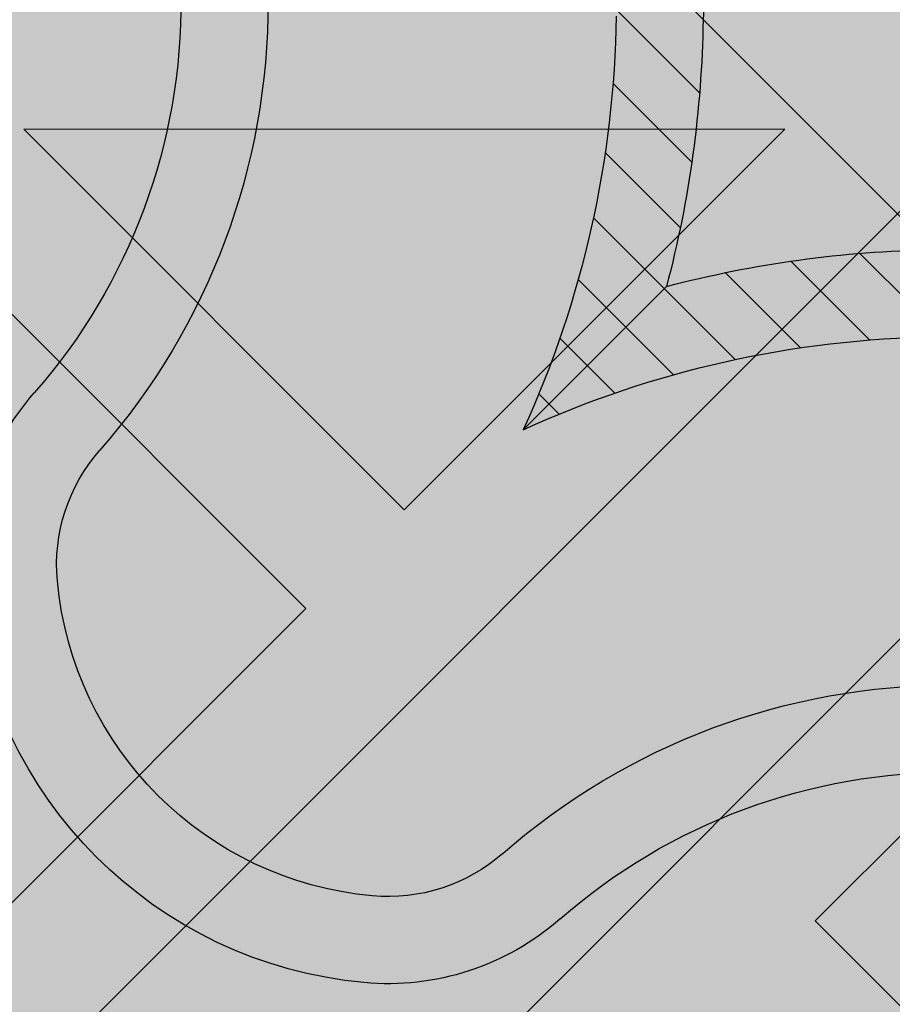
# Model space of a CAD drawing. Units: inches. Extents: x 844 to 2234, y 346 to 1084.
# Tile 70 of 93: x 1999.568 to 2001.166, y 692.525 to 694.327. Entities that reach past the tile are written whole.
import ezdxf

# ---------------------------------------------------------------- set-up
doc = ezdxf.new("R2010")
doc.units = ezdxf.units.IN
doc.header["$MEASUREMENT"] = 0
for name, color, linetype, lineweight in [('A-ANNO-DIMS', 2, 'Continuous', 18), ('furniture', 8, 'Continuous', 18), ('RA-AP-01$0$INT', 35, 'Continuous', 5)]:
    doc.layers.add(name, color=color, linetype=linetype, lineweight=lineweight)
doc.layers.add('RA-AP-01$0$FURN', color=3, linetype='Continuous')
doc.layers.add('RA-AP-01$0$WOOD', color=64, linetype='Continuous')
doc.styles.get("Standard").update_dxf_attribs({"font": 'arial.ttf'})
doc.dimstyles.get("Standard").update_dxf_attribs({"dimtxt": 6, "dimasz": 3, "dimexe": 0.18, "dimexo": 0.0625, "dimgap": 0.09, "dimtad": 0, "dimtih": 1, "dimtoh": 1, "dimdec": 1, "dimzin": 0, "dimdsep": 46, "dimlunit": 3, "dimtxsty": 'Standard', "dimblk": 'ARCHTICK', "dimcen": 0.09, "dimadec": 0, "dimazin": 0, "dimtfac": 1, "dimtdec": 1, "dimtofl": 0, "dimtmove": 0, "dimatfit": 3, "dimfxl": 1, "dimtolj": 1, "dimtzin": 0, "dimarcsym": 0})

# ---------------------------------------------------------------- blocks, each defined once
blk = doc.blocks.new('A$C18D01794')
at = {"layer": 'RA-AP-01$0$INT'}
h = blk.add_hatch(color=256, dxfattribs=at)
h.paths.add_polyline_path([(4.585917135068449, -6.356712009588271), (4.555206456959269, -6.35671200958746), (4.555206456959137, -6.387422687716308), (4.874495778835233, -6.706712009592356), (4.90520645695423, -6.676001331474049)])
h.paths.add_polyline_path([(5.255206456948813, -6.387422687716306), (5.255206456948682, -6.356712009605972), (5.224495778822613, -6.356712009605161), (4.905206456953498, -6.676001331474273), (4.935917135072151, -6.706712009592924)])
h.paths.add_polyline_path([(4.935917135072559, -6.706712009592068), (4.905206456953564, -6.737422687710376), (5.255206456951813, -7.087422687708613), (5.255206456951549, -7.026001331471008)])
h.paths.add_polyline_path([(4.555206456956399, -7.026001331471013), (4.555206456956134, -7.087422687708616), (4.905206456953821, -6.737422687710943), (4.874495778835166, -6.70671200959229)])
h = blk.add_hatch(color=256, dxfattribs=at)
h.paths.add_polyline_path([(4.585917135068448, -6.356712009588273), (4.614201406330596, -6.356712009589021), (4.668846067270487, -6.411356670531338), (4.723490728212344, -6.356712009591912), (4.771774999457151, -6.35671200959319), (4.826419660396886, -6.411356670535356), (4.862780050090322, -6.374996280843536), (4.844495778842715, -6.356712009595112), (4.862780050090411, -6.356712009595595), (4.905206456960182, -6.399138416468211), (4.947632863832445, -6.356712009597838), (4.965917135079675, -6.356712009598322), (4.947632863831759, -6.374996280845421), (4.983993253523576, -6.411356670538857), (5.038637914464627, -6.356712009600247), (5.08692218571208, -6.356712009601523), (5.141566846649976, -6.411356670541852), (5.196211507589851, -6.356712009604411), (5.224495778822615, -6.356712009605161), (4.905206456953975, -6.676001331473793)])
h.paths.add_polyline_path([(4.895206456956031, -6.637717060225675), (4.895206456958921, -6.528427738347902), (4.840561796018589, -6.583072399285802)], flags=16)
h.paths.add_polyline_path([(4.915206456955638, -6.637717060226121), (4.969851117895509, -6.583072399288678), (4.915206456957609, -6.528427738348344)], flags=16)
h.paths.add_polyline_path([(4.826419660395175, -6.568930263661755), (4.881064321335613, -6.514285602723745), (4.771774999456703, -6.514285602720857)], flags=16)
h.paths.add_polyline_path([(4.983993253519558, -6.568930263665262), (5.038637914460456, -6.514285602726792), (4.929348592581548, -6.514285602724816)], flags=16)
h.paths.add_polyline_path([(4.881064321336025, -6.494285602723742), (4.826419660397532, -6.439640941782821), (4.771774999457062, -6.494285602720859)], flags=16)
h.paths.add_polyline_path([(4.929348592582019, -6.494285602724817), (5.038637914460982, -6.494285602726792), (4.983993253522945, -6.439640941786327)], flags=16)
h.paths.add_polyline_path([(4.895206456960191, -6.480143467100443), (4.895206456962115, -6.407422687715913), (4.876922185715016, -6.389138416467584), (4.840561796021581, -6.425498806159401)], flags=16)
h.paths.add_polyline_path([(4.915206456958487, -6.480143467100889), (4.969851117899527, -6.425498806162279), (4.933490728206909, -6.389138416468043), (4.9152064569598, -6.40742268771434)], flags=16)
h.paths.add_polyline_path([(4.757632863832376, -6.480143467096812), (4.812277524772842, -6.425498806158772), (4.757632863834348, -6.370854145217844)], flags=16)
h.paths.add_polyline_path([(4.737632863832376, -6.480143467096286), (4.737632863834348, -6.370854145217375), (4.682988202893906, -6.425498806155385)], flags=16)
h.paths.add_polyline_path([(5.05278005008503, -6.480143467103376), (5.052780050087917, -6.370854145224413), (4.998135389146995, -6.425498806162908)], flags=16)
h.paths.add_polyline_path([(5.072780050085024, -6.480143467103744), (5.127424711025931, -6.42549880616527), (5.072780050087916, -6.370854145224832)], flags=16)
h.paths.add_polyline_path([(4.935917135072783, -6.706712009592292), (5.255206456948811, -6.387422687716309), (5.255206456948932, -6.415706958964177), (5.200561796010279, -6.470351619902839), (5.255206456949403, -6.524996280841948), (5.25520645694961, -6.5732805520894), (5.200561796009787, -6.627925213029239), (5.236922185702417, -6.664285602721864), (5.255206456949919, -6.646001331474357), (5.255206456949998, -6.664285602721898), (5.212780050078687, -6.706712009592262), (5.25520645695036, -6.749138416463932), (5.255206456950438, -6.767422687711313), (5.236922185702424, -6.749138416463297), (5.200561796009796, -6.785498806155928), (5.255206456950753, -6.840143467096874), (5.25520645695096, -6.888427738341682), (5.200561796010322, -6.943072399282328), (5.255206456951428, -6.997717060223427), (5.255206456951547, -7.026001331471006)])
h.paths.add_polyline_path([(5.042988202883395, -6.785498806155427), (5.097632863823085, -6.840143467095101), (5.097632863822622, -6.730854145216193)], flags=16)
h.paths.add_polyline_path([(5.028846067259663, -6.771356670531693), (5.083490728198774, -6.716712009592573), (4.974201406321001, -6.716712009593042)], flags=16)
h.paths.add_polyline_path([(5.117632863823087, -6.840143467095186), (5.172277524762331, -6.785498806155926), (5.11763286382262, -6.730854145216225)], flags=16)
h.paths.add_polyline_path([(5.08349072819877, -6.696712009593886), (5.028846067259652, -6.642067348654775), (4.974201406320998, -6.696712009593438)], flags=16)
h.paths.add_polyline_path([(5.131774999446817, -6.854285602718917), (5.186419660386065, -6.799640941779662), (5.241064321325782, -6.854285602719365)], flags=17)
h.paths.add_polyline_path([(5.131774999446228, -6.716712009592374), (5.186419660386065, -6.771356670532194), (5.222780050079488, -6.734996280838764), (5.204495778832781, -6.716712009592063)], flags=16)
h.paths.add_polyline_path([(5.097632863822613, -6.682569873970264), (5.097632863823061, -6.573280552091354), (5.042988202883383, -6.627925213031044)], flags=16)
h.paths.add_polyline_path([(5.131774999446899, -6.874285602718915), (5.241064321325809, -6.874285602719364), (5.186419660386591, -6.928930263658598)], flags=17)
h.paths.add_polyline_path([(5.131774999446226, -6.696712009594078), (5.204495778830767, -6.696712009594374), (5.22278005007868, -6.67842773834687), (5.186419660386049, -6.642067348654249)], flags=16)
h.paths.add_polyline_path([(5.11763286382262, -6.682569873970225), (5.17227752476232, -6.627925213030515), (5.117632863823064, -6.573280552091267)], flags=16)
h.paths.add_polyline_path([(5.186419660386069, -6.613783077405491), (5.241064321325754, -6.559138416465795), (5.131774999446791, -6.559138416466263)], flags=16)
h.paths.add_polyline_path([(5.131774999446872, -6.539138416466263), (5.24106432132578, -6.539138416465794), (5.186419660386554, -6.484493755526573)], flags=16)
h.paths.add_polyline_path([(5.255206456951811, -7.08742268770861), (5.255206456951895, -7.106712009588038), (4.555206456956052, -7.106712009588038), (4.555206456956136, -7.087422687708617), (4.905206456953973, -6.737422687710788)])
h.paths.add_polyline_path([(4.983993253513404, -6.8444937555241), (4.92934859257295, -6.899138416462108), (5.03863791445186, -6.899138416465014)], flags=16)
h.paths.add_polyline_path([(4.969851117889988, -6.83035161990006), (4.915206456952556, -6.775706958960171), (4.915206456949648, -6.884996280837944)], flags=16)
h.paths.add_polyline_path([(4.929348592572535, -6.919138416462105), (4.983993253511019, -6.973783077403037), (5.038637914451496, -6.919138416465012)], flags=16)
h.paths.add_polyline_path([(5.052780050074912, -6.93328055208906), (4.998135389134438, -6.987925213027088), (5.052780050072919, -7.042569873968025)], flags=16)
h.paths.add_polyline_path([(5.07278005007491, -6.933280552089588), (5.072780050072918, -7.042569873968497), (5.127424711013374, -6.987925213030498)], flags=16)
h.paths.add_polyline_path([(4.89520645695295, -6.775706958959721), (4.840561796013067, -6.830351619897157), (4.895206456950961, -6.884996280837494)], flags=16)
h.paths.add_polyline_path([(4.915206456948365, -6.933280552085403), (4.915206456946434, -7.006001331471951), (4.933490728192729, -7.024285602719066), (4.969851117886972, -6.987925213026453)], flags=16)
h.paths.add_polyline_path([(4.881064321327021, -6.899138416461022), (4.82641966038902, -6.84449375552057), (4.771774999448108, -6.899138416459029)], flags=16)
h.paths.add_polyline_path([(4.895206456950073, -6.933280552084951), (4.840561796009022, -6.987925213023558), (4.876922185700835, -7.024285602716997), (4.895206456948749, -7.006001331469487)], flags=16)
h.paths.add_polyline_path([(4.983993253510392, -7.0020673486505), (4.947632863816944, -7.038427738342319), (4.965917135064043, -7.05671200959023), (5.038637914448995, -7.056712009591555)], flags=16)
h.paths.add_polyline_path([(4.881064321326543, -6.91913841646102), (4.771774999447578, -6.919138416459031), (4.826419660385607, -6.973783077399508)], flags=16)
h.paths.add_polyline_path([(4.905206456946447, -7.014285602717636), (4.862780050074785, -7.056712009588352), (4.947632863816685, -7.056712009589775)], flags=16)
h.paths.add_polyline_path([(5.14156684663679, -7.002067348654549), (5.086922185696452, -7.056712009592438), (5.196211507574223, -7.056712009594425)], flags=16)
h.paths.add_polyline_path([(4.8264196603837, -7.002067348646972), (4.771774999442643, -7.056712009585575), (4.8444957788276, -7.056712009587508), (4.862780050075511, -7.038427738340416)], flags=16)
h.paths.add_polyline_path([(4.812277524760289, -6.98792521302292), (4.757632863822258, -6.933280552082447), (4.757632863819352, -7.042569873961408)], flags=16)
h.paths.add_polyline_path([(4.73763286382226, -6.933280552082079), (4.682988202881349, -6.987925213020536), (4.737632863819352, -7.04256987396099)], flags=16)
h.paths.add_polyline_path([(4.723490728195188, -7.056712009584289), (4.668846067257299, -7.002067348643949), (4.614201406317417, -7.056712009581383)], flags=16)
h.paths.add_polyline_path([(4.597632863829262, -6.706712009592262), (4.555206456957951, -6.664285602721896), (4.555206456958029, -6.646001331474357), (4.573490728205535, -6.664285602721864), (4.609851117898167, -6.627925213029238), (4.555206456958338, -6.573280552089402), (4.555206456958546, -6.524996280841952), (4.60985111789767, -6.470351619902839), (4.555206456959015, -6.415706958964177), (4.555206456959138, -6.387422687716309), (4.874495778835167, -6.70671200959229), (4.5552064569564, -7.026001331471015), (4.555206456956523, -6.997717060223433), (4.609851117897629, -6.94307239928233), (4.555206456956988, -6.888427738341681), (4.555206456957198, -6.840143467096881), (4.609851117898153, -6.78549880615593), (4.573490728205528, -6.749138416463297), (4.555206456957507, -6.76742268771132), (4.555206456957585, -6.749138416463933)])
h.paths.add_polyline_path([(4.712780050085332, -6.730854145216195), (4.712780050084863, -6.840143467095105), (4.767424711024555, -6.785498806155427)], flags=16)
h.paths.add_polyline_path([(4.726922185709173, -6.716712009592573), (4.781566846648288, -6.771356670531693), (4.836211507586949, -6.716712009593043)], flags=16)
h.paths.add_polyline_path([(4.692780050085327, -6.730854145216225), (4.638135389145619, -6.785498806155928), (4.692780050084865, -6.840143467095185)], flags=16)
h.paths.add_polyline_path([(4.726922185709182, -6.696712009593886), (4.836211507586949, -6.696712009593436), (4.7815668466483, -6.642067348654773)], flags=16)
h.paths.add_polyline_path([(4.678637914461726, -6.71671200959237), (4.605917135075169, -6.716712009592063), (4.587632863828464, -6.734996280838766), (4.623993253521887, -6.771356670532195)], flags=16)
h.paths.add_polyline_path([(4.712780050085336, -6.68256987397026), (4.767424711024568, -6.627925213031042), (4.71278005008489, -6.573280552091352)], flags=16)
h.paths.add_polyline_path([(4.678637914461726, -6.696712009594076), (4.623993253521899, -6.642067348654247), (4.587632863829271, -6.67842773834687), (4.605917135077185, -6.696712009594376)], flags=16)
h.paths.add_polyline_path([(4.692780050085336, -6.682569873970228), (4.692780050084889, -6.573280552091267), (4.638135389145632, -6.627925213030515)], flags=16)
h.paths.add_polyline_path([(4.623993253521885, -6.799640941779662), (4.678637914461131, -6.854285602718915), (4.56934859258217, -6.854285602719365)], flags=17)
h.paths.add_polyline_path([(4.623993253521901, -6.613783077405509), (4.678637914461158, -6.559138416466263), (4.569348592582195, -6.559138416465795)], flags=16)
h.paths.add_polyline_path([(4.678637914461051, -6.874285602718915), (4.623993253521361, -6.928930263658598), (4.569348592582143, -6.874285602719364)], flags=17)
h.paths.add_polyline_path([(4.678637914461076, -6.539138416466263), (4.623993253521399, -6.484493755526573), (4.569348592582167, -6.539138416465796)], flags=16)
h = blk.add_hatch(color=256, dxfattribs=at)
h.paths.add_polyline_path([(4.969851117891331, -6.583072399286455), (4.915206456952669, -6.63771706022511), (4.915206456952222, -6.528427738347337)])
h.paths.add_polyline_path([(4.895206456953064, -6.637717060225108), (4.840561796014413, -6.583072399286448), (4.895206456953533, -6.528427738347335)])
h.paths.add_polyline_path([(4.826419660390684, -6.568930263662714), (4.771774999451003, -6.514285602723024), (4.881064321329913, -6.514285602723489)])
h.paths.add_polyline_path([(4.881064321329884, -6.494285602723492), (4.771774999450921, -6.494285602723024), (4.82641966039018, -6.439640941783778)])
h.paths.add_polyline_path([(4.895206456953734, -6.48014346709988), (4.840561796013912, -6.425498806160046), (4.876922185707337, -6.389138416466622), (4.895206456954043, -6.40742268771333)])
h.paths.add_polyline_path([(4.862780050082808, -6.374996280843689), (4.826419660390178, -6.411356670536314), (4.771774999450351, -6.356712009596481), (4.844495778835303, -6.356712009596181)])
h.paths.add_polyline_path([(4.812277524766446, -6.425498806160041), (4.757632863827191, -6.480143467099289), (4.757632863826741, -6.370854145220329)])
h.paths.add_polyline_path([(4.737632863827191, -6.480143467099214), (4.682988202887508, -6.425498806159518), (4.737632863826743, -6.370854145220299)])
h.paths.add_polyline_path([(4.668846067263777, -6.41135667053579), (4.614201406325123, -6.356712009597128), (4.723490728202894, -6.356712009596675)])
h.paths.add_polyline_path([(4.905206456953846, -6.399138416467422), (4.862780050082654, -6.356712009596229), (4.947632863824561, -6.356712009595756)])
h.paths.add_polyline_path([(4.915206456952028, -6.480143467099882), (4.91520645695173, -6.407422687715346), (4.933490728199234, -6.389138416467428), (4.96985111789186, -6.425498806160055)])
h.paths.add_polyline_path([(5.038637914454841, -6.494285602723048), (4.929348592575874, -6.494285602723497), (4.983993253515593, -6.439640941783787)])
h.paths.add_polyline_path([(4.983993253515065, -6.568930263662725), (4.929348592575849, -6.514285602723495), (5.038637914454755, -6.514285602723045)])
h.paths.add_polyline_path([(5.052780050079843, -6.480143467099317), (4.998135389140595, -6.425498806160058), (5.052780050080309, -6.370854145220356)])
h.paths.add_polyline_path([(4.983993253516868, -6.411356670536324), (4.947632863824241, -6.374996280843694), (4.965917135071747, -6.356712009596188), (5.038637914456701, -6.356712009596504)])
h.paths.add_polyline_path([(5.127424711019533, -6.425498806159557), (5.072780050079843, -6.480143467099239), (5.07278005008031, -6.370854145220326)])
h.paths.add_polyline_path([(5.141566846643269, -6.411356670535829), (5.086922185704154, -6.356712009596707), (5.196211507581929, -6.356712009597176)])
h = blk.add_hatch(color=256, dxfattribs=at)
h.paths.add_polyline_path([(5.028846067259997, -6.642067348655121), (4.974201406321342, -6.696712009593783), (5.083490728199115, -6.69671200959423)])
h.paths.add_polyline_path([(4.974201406321344, -6.716712009593388), (5.028846067260004, -6.771356670532039), (5.083490728199117, -6.716712009592919)])
h.paths.add_polyline_path([(5.042988202883738, -6.785498806155768), (5.097632863823428, -6.840143467095449), (5.097632863822963, -6.73085414521654)])
h.paths.add_polyline_path([(5.117632863822961, -6.730854145216568), (5.117632863823428, -6.840143467095531), (5.172277524762674, -6.785498806156272)])
h.paths.add_polyline_path([(5.131774999446572, -6.716712009592718), (5.186419660386406, -6.77135667053254), (5.222780050079831, -6.734996280839116), (5.204495778833122, -6.716712009592409)])
h.paths.add_polyline_path([(5.236922185702764, -6.749138416463644), (5.200561796010139, -6.785498806156274), (5.255206456949971, -6.840143467096101), (5.255206456950271, -6.76742268771115)])
h.paths.add_polyline_path([(5.186419660386412, -6.799640941780006), (5.131774999447164, -6.854285602719262), (5.241064321326123, -6.854285602719711)])
h.paths.add_polyline_path([(5.131774999447238, -6.874285602719261), (5.186419660386934, -6.928930263658944), (5.241064321326153, -6.874285602719709)])
h.paths.add_polyline_path([(5.200561796010663, -6.943072399282675), (5.255206456949324, -6.997717060221329), (5.255206456949777, -6.888427738343558)])
h.paths.add_polyline_path([(5.21278005007903, -6.706712009592607), (5.255206456950223, -6.749138416463798), (5.255206456950696, -6.664285602721891)])
h.paths.add_polyline_path([(5.13177499944657, -6.696712009594424), (5.204495778831106, -6.696712009594723), (5.222780050079024, -6.678427738347219), (5.186419660386397, -6.642067348654592)])
h.paths.add_polyline_path([(5.117632863823405, -6.573280552091611), (5.117632863822955, -6.682569873970578), (5.172277524762665, -6.627925213030859)])
h.paths.add_polyline_path([(5.042988202883727, -6.627925213031387), (5.097632863822957, -6.682569873970603), (5.097632863823407, -6.573280552091697)])
h.paths.add_polyline_path([(5.131774999447135, -6.559138416466609), (5.186419660386394, -6.613783077405857), (5.241064321326097, -6.559138416466144)])
h.paths.add_polyline_path([(5.200561796010128, -6.627925213029584), (5.236922185702758, -6.664285602722211), (5.255206456950264, -6.646001331474705), (5.255206456949948, -6.573280552089752)])
h.paths.add_polyline_path([(5.186419660386895, -6.484493755526919), (5.131774999447213, -6.539138416466609), (5.241064321326127, -6.539138416466142)])
h.paths.add_polyline_path([(5.200561796010624, -6.470351619903183), (5.255206456949745, -6.524996280842298), (5.255206456949276, -6.415706958964523)])
for p, q in [((4.905206456953975, -6.676001331473793), (5.224495778822613, -6.356712009605161)), ((5.072780050087916, -6.37085414522483), (5.127424711025931, -6.42549880616527)), ((4.935917135072783, -6.706712009592292), (5.255206456948813, -6.387422687716307)), ((5.255206456948934, -6.415706958964177), (5.200561796010281, -6.470351619902839)), ((5.12742471102593, -6.425498806165272), (5.072780050085028, -6.48014346710374)), ((5.255206456949399, -6.524996280841946), (5.200561796010281, -6.470351619902839)), ((5.18641966038655, -6.484493755526575), (5.131774999446872, -6.539138416466263)), ((5.241064321325782, -6.539138416465796), (5.186419660386552, -6.484493755526573)), ((5.131774999446872, -6.539138416466263), (5.241064321325782, -6.539138416465796))]:
    blk.add_line(p, q, dxfattribs=at)
blk = doc.blocks.new('A$C32926AE1')
at = {"layer": 'RA-AP-01$0$WOOD'}
h = blk.add_hatch(color=256, dxfattribs=at)
h.dxf.hatch_style = 1
h.paths.add_polyline_path([(5.157430609644524, 4.573483066760929, -0.1009492694046607), (5.155401577623758, 4.593365984175333, -0.1842662638101597), (5.172249623284174, 4.638795604568598, 0.2056608120311276), (5.179560981299304, 4.661316324430096, 0.3614336704623542), (5.134352340494423, 4.706524965234944, 0.2056608120311297), (5.111831620632933, 4.699213607219793, -0.1842662638101113), (5.066402000239693, 4.682365561559342, -0.1055311479399994), (5.045656153913092, 4.68467289944697, 0.1567636581983829), (4.763886414745334, 4.684672899446966, -0.1055311479399895), (4.743140568418733, 4.68236556155934, -0.1842662638100833), (4.6977109480255, 4.69921360721979, 0.2056608120302612), (4.675190228164109, 4.706524965234949, 0.3614336704708441), (4.629981587358889, 4.66131632442871, 0.2056608120245944), (4.637292945374126, 4.638795604567974, -0.1842662638101024), (4.654140991034615, 4.59336598417475, -0.1009492694055169), (4.652111959013835, 4.573483066760181, 0.021410119221476), (4.629748025606143, 4.156712009541676, 0.0214101192214795), (4.652111959013809, 3.739940952323101, -0.1009492694059586), (4.654140991034615, 3.720058034908448, -0.1842662638100975), (4.637292945374126, 3.674628414515226, 0.2056608120245705), (4.629981587358889, 3.652107694654492, 0.3614336704708879), (4.675190228164113, 3.606899053848249, 0.2056608120302384), (4.697710948025501, 3.614210411863408, -0.1842662638100995), (4.743140568418738, 3.63105845752386, -0.1055311479402541), (4.763886414745388, 3.628751119636215, 0.1567636581983776), (5.045656153913137, 3.628751119636244, -0.1055311479397538), (5.066402000239692, 3.631058457523857, -0.1842662638101067), (5.111831620632931, 3.614210411863407, 0.2056608120310924), (5.134352340494417, 3.606899053848256, 0.3614336704624001), (5.179560981299307, 3.652107694653103, 0.2056608120311314), (5.172249623284175, 3.6746284145146, -0.1842662638101402), (5.155401577623758, 3.72005803490786, -0.1009492694051366), (5.15743060964455, 3.739940952322354, 0.0214101192215073), (5.179794543052287, 4.156712009541468, 0.0214101192215252)])
h.paths.add_polyline_path([(4.639748609479751, 4.156712009541513, 0.0213537860821624), (4.661970494867118, 3.741887061152232, -0.094075836301374), (4.664143710413708, 3.7196126951003, -0.1824818158568985), (4.644813765429836, 3.668037719127816, 0.2056608120245319), (4.639939526753007, 3.653023905887301, 0.3614336704710246), (4.676106439397173, 3.616856993242342, 0.2056608120302234), (4.691120252638095, 3.621731231919122, -0.1824818158602558), (4.742695228611606, 3.641061176902986, -0.1029891339458722), (4.766991894714349, 3.638256818950944, 0.156709409989566), (5.042550673941472, 3.638256818950105, -0.102989133958497), (5.066847340047078, 3.641061176902949, -0.1824818158594995), (5.118422316020358, 3.621731231919103, 0.2056608120311416), (5.133436129261316, 3.616856993242346, 0.3614336704621468), (5.169603041905217, 3.653023905886178, 0.2056608120310986), (5.164728803228477, 3.668037719127177, -0.1824818158565612), (5.145398858244737, 3.719612695099578, -0.0940758363009313), (5.147572073791232, 3.741887061151398, 0.0213537860822023), (5.169793959178681, 4.156712009541451, 0.0213537860822226), (5.147572073791203, 4.571536957931898, -0.0940758363005034), (5.145398858244737, 4.59381132398362, -0.1824818158565587), (5.164728803228476, 4.645386299956021, 0.2056608120311045), (5.169603041905216, 4.66040011319702, 0.3614336704621845), (5.133436129261313, 4.696567025840856, 0.2056608120310773), (5.118422316020359, 4.691692787164098, -0.182481815859508), (5.066847340047078, 4.67236284218025, -0.1029891339584606), (5.04255067394148, 4.675167200133092, 0.156709409989566), (4.766991894714357, 4.675167200132257, -0.1029891339458842), (4.742695228611611, 4.672362842180213, -0.1824818158602725), (4.691120252638095, 4.691692787164077, 0.2056608120302152), (4.676106439397174, 4.696567025840858, 0.3614336704710363), (4.639939526753005, 4.660400113195899, 0.2056608120245495), (4.644813765429837, 4.645386299955384, -0.1824818158568934), (4.664143710413708, 4.593811323982902, -0.0940758363009187), (4.661970494867149, 4.571536957931074, 0.021353786082177)], flags=16)
h.paths.add_polyline_path([(5.129794543052235, 4.432167055276933, -0.0141661062790638), (5.130152669293814, 4.156927903047693, -0.0141661062790647), (5.129794543052234, 3.881688750818433, -0.0785247771143638), (5.10979738006795, 3.755143611847103, 0.0945969212073497), (5.105408519571111, 3.717898134952927, 0.1043170707844957), (5.116074640131521, 3.670385395016088, 0.1043170707864965), (5.068561900193738, 3.681051515576561, 0.09459692119553), (5.031316423304057, 3.676662655080835, -0.1580239521427272), (4.778226145355827, 3.676662655080367, 0.0945969211986668), (4.740980668464973, 3.681051515576592, 0.1043170707882822), (4.693467928526415, 3.670385395015844, 0.1043170707867916), (4.704134049087309, 3.717898134953662, 0.0945969211972894), (4.69974518859162, 3.755143611844042, -0.0785247771163196), (4.679748025606343, 3.881688750818406, -0.0141661062790663), (4.679389899364763, 4.156927903047693, -0.0141661062790672), (4.679748025606343, 4.432167055276998, -0.0785247771163064), (4.699745188591625, 4.55871219425134, 0.094596921197333), (4.704134049087308, 4.595957671141738, 0.1043170707867205), (4.693467928526416, 4.643470411079523, 0.1043170707882628), (4.740980668464965, 4.632804290518776, 0.0945969211988114), (4.778226145355874, 4.637193151015016, -0.158023952142669), (5.031316423304015, 4.637193151014546, 0.0945969211956361), (5.068561900193736, 4.632804290518806, 0.1043170707864979), (5.11607464013152, 4.643470411079278, 0.1043170707844617), (5.105408519571112, 4.595957671142455, 0.0945969212074597), (5.109797380067959, 4.558712194248236, -0.0785247771143467)], flags=0)
h.paths.add_polyline_path([(5.119794532311105, 4.432259799204851, -0.0142000800617244), (5.120156169157484, 4.156927903047701, -0.0142000800617277), (5.119794532311105, 3.881596006890482, -0.0784894509520253), (5.100273383573699, 3.758192358677797, 0.0940138827242913), (5.095413455884425, 3.717477693979438, 0.0606271852308753), (5.099615656341024, 3.686844378806616, 0.0606271852322524), (5.068982341167493, 3.691046579263239, 0.0940138827010453), (5.028267676478798, 3.686186651576848, -0.1580706864508061), (4.781274892180912, 3.686186651576435, 0.0940138827026903), (4.740560227491556, 3.691046579263279, 0.0606271852339895), (4.709926912317155, 3.686844378806508, 0.0606271852329405), (4.714129112773991, 3.717477693980356, 0.094013882701304), (4.709269185087677, 3.758192358669163, -0.0784894509577193), (4.689748036347473, 3.881596006890469, -0.014200080061729), (4.689386399501094, 4.156927903047709, -0.0142000800617217), (4.689748036347473, 4.432259799204808, -0.078489450957724), (4.709269185087651, 4.555663447426125, 0.0940138827014585), (4.714129112773992, 4.596378112114996, 0.0606271852329731), (4.709926912317154, 4.62701142728886, 0.0606271852340196), (4.74056022749157, 4.622809226832087, 0.0940138827024997), (4.781274892180847, 4.627669154518912, -0.1580706864508359), (5.028267676478777, 4.627669154518526, 0.0940138827010946), (5.068982341167492, 4.622809226832129, 0.060627185232254), (5.099615656341024, 4.627011427288751, 0.0606271852308727), (5.095413455884425, 4.59637811211593, 0.0940138827241088), (5.100273383573675, 4.555663447417647, -0.0784894509520978)], flags=0)
h.paths.add_polyline_path([(5.06978912287499, 4.430218106756144, -0.014241683694547), (5.070173729147532, 4.156927903047672, -0.0142416836945458), (5.06978912287499, 3.883637699339223, -0.0800609523125196), (5.052662118612511, 3.773463122773442, 0.0526421978001116), (5.04590916754064, 3.740550867606997, 0.0526421977992423), (5.012996912374707, 3.73379791653534, -0.1583028414718258), (4.796545656286308, 3.73379791653451, 0.0526421978034211), (4.763633401117837, 3.740550867607021, 0.0526421978018622), (4.756880450045755, 3.773463122774558, -0.0800609523117106), (4.739753445783639, 3.883637699339268, -0.0142416836945435), (4.739368839511098, 4.156927903047671, -0.0142416836945477), (4.739753445783639, 4.430218106756155, -0.0800609523116345), (4.75688045004574, 4.540392683320762, 0.052642197801941), (4.763633401117837, 4.573304938488346, 0.0526421978035071), (4.796545656286361, 4.580057889560873, -0.1583028414717561), (5.012996912374669, 4.580057889560039, 0.0526421977993048), (5.04590916754064, 4.57330493848837, 0.0526421978002057), (5.052662118612529, 4.540392683321868, -0.080060952312477)], flags=0)
h.paths.add_polyline_path([(5.049789715110557, 4.43038092723357, -0.0143097550741839), (5.05018085590259, 4.156927903047715, -0.0143097550741854), (5.049789715110558, 3.883474878861827, -0.0800685599149176), (5.03362098255317, 3.779581877367999, 0.0306258898956367), (5.028241146483733, 3.758218888663947, 0.0306258898977031), (5.006878157778253, 3.75283905259408, -0.1583983521624096), (4.802664410878162, 3.752839052594731, 0.0306258898946014), (4.781301422174808, 3.758218888663924, 0.0306258898967912), (4.775921586105202, 3.779581877368794, -0.080068559914251), (4.759752853548071, 3.883474878861786, -0.0143097550741854), (4.759361712756037, 4.156927903047671, -0.0143097550741854), (4.759752853548071, 4.430380927233557, -0.0800685599142479), (4.775921586105193, 4.534273928726546, 0.0306258898968306), (4.781301422174808, 4.555636917431444, 0.0306258898945754), (4.802664410878143, 4.561016753500631, -0.1583983521624168), (5.006878157778244, 4.561016753501291, 0.0306258898977177), (5.028241146483733, 4.555636917431421, 0.0306258898958182), (5.03362098255321, 4.534273928727244, -0.080068559914796)], flags=0)
h.paths.add_polyline_path([(4.999766070382627, 4.428171244713864, -0.0143443147609634), (5.000198441819402, 4.156927903047689, -0.0143443147609612), (4.999766070382627, 3.885684561381556, -0.0784641635803329), (4.987356730658798, 3.799103304488872, -0.1506053783831347), (4.822185837999821, 3.79910330448882, -0.0784641635803318), (4.809776498276007, 3.885684561381509, -0.014344314760963), (4.809344126839227, 4.156927903047677, -0.0143443147609645), (4.809776498276007, 4.428171244713873, -0.0784641635803192), (4.822185837999822, 4.514752501606549, -0.1506053783831338), (4.987356730658798, 4.514752501606494, -0.078464163580285)], flags=0)
h.paths.add_polyline_path([(4.979755254238824, 4.42764379880488, -0.0143772539198268), (4.980205517789977, 4.156927903047693, -0.0143772539198275), (4.979755254238824, 3.886212007290489, -0.0689242507424422), (4.971183264704897, 3.815276770442801, -0.1296645318904179), (4.838359303953726, 3.815276770442746, -0.0689242507424186), (4.829787314419809, 3.886212007290419, -0.0143772539198292), (4.829337050868653, 4.156927903047653, -0.0143772539198325), (4.829787314419809, 4.427643798804946, -0.0689242507424211), (4.838359303953725, 4.498579035652621, -0.1296645318904187), (4.971183264704897, 4.498579035652565, -0.0689242507424401)], flags=0)
h = blk.add_hatch(color=256, dxfattribs=at)
h.dxf.hatch_style = 1
h.paths.add_polyline_path([(5.145398858244737, 4.59381132398362, -0.1824818158565616), (5.164728803228476, 4.645386299956021, 0.2056608120311045), (5.169603041905216, 4.66040011319702, 0.3614336704621845), (5.133436129261313, 4.696567025840856, 0.2056608120310773), (5.118422316020359, 4.691692787164098, -0.182481815859508), (5.066847340047078, 4.67236284218025, -0.1029891339584606), (5.04255067394148, 4.675167200133092, 0.156709409989566), (4.766991894714357, 4.675167200132257, -0.1029891339458842), (4.742695228611611, 4.672362842180213, -0.1824818158602725), (4.691120252638095, 4.691692787164077, 0.2056608120302152), (4.676106439397174, 4.696567025840858, 0.3614336704710363), (4.639939526753005, 4.660400113195899, 0.2056608120245495), (4.644813765429837, 4.645386299955384, -0.1824818158568934), (4.664143710413708, 4.593811323982902, -0.0940758363009187), (4.661970494867149, 4.571536957931074, 0.0213537860821772), (4.639748609479751, 4.156712009541507, 0.0213537860821625), (4.661970494867119, 3.741887061152226, -0.0940758363013071), (4.664143710413708, 3.719612695100309, -0.1824818158569294), (4.644813765429836, 3.668037719127816, 0.2056608120245319), (4.639939526753007, 3.653023905887301, 0.3614336704710246), (4.676106439397173, 3.616856993242342, 0.2056608120302234), (4.691120252638095, 3.621731231919122, -0.1824818158602558), (4.742695228611606, 3.641061176902986, -0.1029891339458722), (4.766991894714349, 3.638256818950944, 0.156709409989566), (5.042550673941472, 3.638256818950105, -0.102989133958497), (5.066847340047078, 3.641061176902949, -0.1824818158594995), (5.118422316020358, 3.621731231919103, 0.2056608120311416), (5.133436129261316, 3.616856993242346, 0.3614336704621468), (5.169603041905217, 3.653023905886178, 0.2056608120310986), (5.164728803228477, 3.668037719127177, -0.1824818158565612), (5.145398858244737, 3.719612695099578, -0.0940758363009313), (5.147572073791232, 3.741887061151398, 0.0213537860822023), (5.169793959178681, 4.156712009541451, 0.0213537860822226), (5.147572073791203, 4.571536957931898, -0.0940758363004996)])
h.paths.add_polyline_path([(5.109797380067958, 4.55871219424824, -0.0785247771143472), (5.129794543052234, 4.432167055276936, -0.0141661062790644), (5.130152669293814, 4.156927903047685, -0.014166106279066), (5.129794543052234, 3.881688750818401, -0.0785247771143517), (5.109797380067946, 3.755143611847092, 0.0945969212073132), (5.105408519571111, 3.717898134952929, 0.1043170707844995), (5.116074640131521, 3.670385395016088, 0.1043170707864965), (5.068561900193738, 3.681051515576561, 0.09459692119553), (5.031316423304057, 3.676662655080835, -0.1580239521427272), (4.778226145355827, 3.676662655080367, 0.0945969211986668), (4.740980668464973, 3.681051515576592, 0.1043170707882822), (4.693467928526415, 3.670385395015844, 0.1043170707867916), (4.704134049087309, 3.717898134953662, 0.0945969211972894), (4.69974518859162, 3.755143611844042, -0.0785247771163196), (4.679748025606343, 3.881688750818406, -0.0141661062790663), (4.679389899364763, 4.156927903047693, -0.0141661062790672), (4.679748025606343, 4.432167055276998, -0.0785247771163064), (4.699745188591625, 4.55871219425134, 0.094596921197333), (4.704134049087308, 4.595957671141738, 0.1043170707867205), (4.693467928526416, 4.643470411079523, 0.1043170707882628), (4.740980668464965, 4.632804290518776, 0.0945969211988114), (4.778226145355874, 4.637193151015016, -0.158023952142669), (5.031316423304015, 4.637193151014546, 0.0945969211956361), (5.068561900193736, 4.632804290518806, 0.1043170707864979), (5.11607464013152, 4.643470411079278, 0.1043170707844617), (5.105408519571112, 4.595957671142455, 0.0945969212074504)], flags=16)
h.paths.add_polyline_path([(5.100273383573655, 4.55566344741771, -0.0784894509521388), (5.119794532311105, 4.432259799204852, -0.0142000800617252), (5.120156169157484, 4.156927903047686, -0.014200080061726), (5.119794532311105, 3.881596006890502, -0.0784894509520446), (5.100273383573696, 3.758192358677786, 0.0940138827242721), (5.095413455884425, 3.717477693979436, 0.0606271852308692), (5.099615656341024, 3.686844378806616, 0.0606271852322522), (5.068982341167493, 3.691046579263239, 0.0940138827010453), (5.028267676478798, 3.686186651576848, -0.1580706864508061), (4.781274892180912, 3.686186651576435, 0.0940138827026903), (4.740560227491556, 3.691046579263279, 0.0606271852339895), (4.709926912317155, 3.686844378806508, 0.0606271852329405), (4.714129112773991, 3.717477693980356, 0.094013882701304), (4.709269185087677, 3.758192358669163, -0.0784894509577193), (4.689748036347473, 3.881596006890469, -0.014200080061729), (4.689386399501094, 4.156927903047709, -0.0142000800617217), (4.689748036347473, 4.432259799204808, -0.078489450957724), (4.709269185087651, 4.555663447426125, 0.0940138827014585), (4.714129112773992, 4.596378112114996, 0.0606271852329731), (4.709926912317154, 4.62701142728886, 0.0606271852340196), (4.74056022749157, 4.622809226832087, 0.0940138827024997), (4.781274892180847, 4.627669154518912, -0.1580706864508359), (5.028267676478777, 4.627669154518526, 0.0940138827010946), (5.068982341167492, 4.622809226832129, 0.060627185232254), (5.099615656341024, 4.627011427288751, 0.0606271852308727), (5.095413455884425, 4.59637811211593, 0.094013882723957)], flags=0)
h.paths.add_polyline_path([(5.04590916754064, 4.57330493848837, 0.0526421978002057), (5.052662118612529, 4.540392683321868, -0.0800609523124783), (5.06978912287499, 4.430218106756142, -0.0142416836945469), (5.070173729147532, 4.156927903047672, -0.0142416836945458), (5.06978912287499, 3.883637699339223, -0.0800609523125196), (5.052662118612511, 3.773463122773442, 0.0526421978001116), (5.04590916754064, 3.740550867606997, 0.0526421977992423), (5.012996912374707, 3.73379791653534, -0.1583028414718258), (4.796545656286308, 3.73379791653451, 0.0526421978034211), (4.763633401117837, 3.740550867607021, 0.0526421978018622), (4.756880450045755, 3.773463122774558, -0.0800609523117106), (4.739753445783639, 3.883637699339268, -0.0142416836945435), (4.739368839511098, 4.156927903047671, -0.0142416836945477), (4.739753445783639, 4.430218106756155, -0.0800609523116345), (4.75688045004574, 4.540392683320762, 0.052642197801941), (4.763633401117837, 4.573304938488346, 0.0526421978035071), (4.796545656286361, 4.580057889560873, -0.1583028414717561), (5.012996912374669, 4.580057889560039, 0.0526421977993048)], flags=0)
h.paths.add_polyline_path([(5.028241146483733, 4.555636917431422, 0.0306258898956949), (5.033620982553182, 4.534273928727329, -0.0800685599148649), (5.049789715110557, 4.430380927233569, -0.0143097550741839), (5.05018085590259, 4.156927903047715, -0.0143097550741854), (5.049789715110558, 3.883474878861827, -0.0800685599149176), (5.03362098255317, 3.779581877367999, 0.0306258898956367), (5.028241146483733, 3.758218888663947, 0.0306258898977031), (5.006878157778253, 3.75283905259408, -0.1583983521624096), (4.802664410878162, 3.752839052594731, 0.0306258898946014), (4.781301422174808, 3.758218888663924, 0.0306258898967912), (4.775921586105202, 3.779581877368794, -0.080068559914251), (4.759752853548071, 3.883474878861786, -0.0143097550741854), (4.759361712756037, 4.156927903047671, -0.0143097550741854), (4.759752853548071, 4.430380927233557, -0.0800685599142479), (4.775921586105193, 4.534273928726546, 0.0306258898968306), (4.781301422174808, 4.555636917431444, 0.0306258898945754), (4.802664410878143, 4.561016753500631, -0.1583983521624168), (5.006878157778244, 4.561016753501291, 0.0306258898977174)], flags=0)
h.paths.add_polyline_path([(4.987356730658798, 4.514752501606494, -0.0784641635803018), (4.999766070382627, 4.428171244713845, -0.0143443147609637), (5.000198441819402, 4.156927903047665, -0.0143443147609622), (4.999766070382628, 3.885684561381514, -0.0784641635802952), (4.987356730658797, 3.799103304488872, -0.1506053783831338), (4.822185837999821, 3.799103304488819, -0.0784641635803342), (4.809776498276007, 3.885684561381512, -0.0143443147609628), (4.809344126839227, 4.156927903047676, -0.0143443147609646), (4.809776498276007, 4.428171244713873, -0.0784641635803192), (4.822185837999822, 4.514752501606549, -0.1506053783831338)], flags=0)
h.paths.add_polyline_path([(4.971183264704897, 4.498579035652566, -0.0689242507424384), (4.979755254238824, 4.427643798804883, -0.0143772539198276), (4.980205517789977, 4.15692790304768, -0.0143772539198258), (4.979755254238823, 3.88621200729051, -0.0689242507424628), (4.971183264704897, 3.815276770442801, -0.129664531890417), (4.838359303953726, 3.815276770442746, -0.0689242507424186), (4.829787314419809, 3.886212007290419, -0.0143772539198292), (4.829337050868653, 4.156927903047653, -0.0143772539198325), (4.829787314419809, 4.427643798804946, -0.0689242507424211), (4.838359303953725, 4.498579035652621, -0.1296645318904187)], flags=0)
h = blk.add_hatch(dxfattribs=at)
h.set_pattern_fill('ANSI31', color=256, scale=0.05, style=0)
h.set_pattern_definition([(45, (0, 0), (-0.0044194173824159, 0.0044194173824159), [])])
h.paths.add_polyline_path([(5.130152669293814, 4.156927903047704, 0.0141661062790657), (5.129794543052234, 4.432167055276982, 0.0777827904001433), (5.110168979996553, 4.557559993161921, -0.0976515123401879), (5.105408519571111, 4.595957671142454, -0.1043170707844687), (5.116074640131522, 4.64347041107928), (5.099615656341024, 4.627011427288751, 0.0606271852308727), (5.095413455884425, 4.59637811211593, 0.0940138827241088), (5.100273383573675, 4.555663447417647, -0.0784894509520972), (5.119794532311105, 4.432259799204852, -0.0142000800617252), (5.120156169157484, 4.156927903047686, -0.014200080061726), (5.119794532311105, 3.881596006890502, -0.0784894509520446), (5.100273383573696, 3.758192358677786, 0.0940138827242721), (5.095413455884425, 3.717477693979436, 0.0606271852308692), (5.099615656341024, 3.686844378806616), (5.116074640131519, 3.67038539501609, -0.1043170707844594), (5.105408519571112, 3.717898134952912, -0.0976515123401594), (5.11016897999655, 3.756295812933435, 0.0777827904001654), (5.129794543052234, 3.881688750818409, 0.0141661062790665)])
h.paths.add_polyline_path([(5.030164222210597, 3.676291055149937, -0.0976515123472002), (5.068561900193739, 3.681051515576561, -0.1043170707864927), (5.116074640131521, 3.670385395016088), (5.099615656341024, 3.686844378806616, 0.0606271852322522), (5.068982341167493, 3.691046579263239, 0.0940138827010453), (5.028267676478798, 3.686186651576848, -0.1580706864508061), (4.781274892180912, 3.686186651576435, 0.0940138827026903), (4.740560227491556, 3.691046579263279, 0.0606271852339913), (4.709926912317154, 3.686844378806508), (4.693467928526416, 3.670385395015845, -0.1043170707882796), (4.740980668464973, 3.681051515576592, -0.0976515123427246), (4.779378346446416, 3.676291055150394, 0.156512506893803)])
h.paths.add_polyline_path([(4.689748036347473, 3.881596006890472, -0.014200080061729), (4.689386399501094, 4.156927903047712, -0.0142000800617195), (4.689748036347473, 4.432259799204768, -0.078489450957742), (4.709269185087648, 4.555663447426114, 0.0940138827014821), (4.714129112773992, 4.596378112114995, 0.0606271852329748), (4.709926912317154, 4.62701142728886), (4.693467928526414, 4.643470411079524, -0.1043170707867939), (4.704134049087309, 4.595957671141706, -0.09765151234893), (4.699373588660725, 4.557559993157876, 0.0777827903975372), (4.679748025606343, 4.432167055276987, 0.0141661062790675), (4.679389899364763, 4.156927903047675, 0.0141661062790641), (4.679748025606343, 3.88168875081843, 0.0777827903975637), (4.699373588660724, 3.756295812937497, -0.0976515123490278), (4.704134049087308, 3.717898134953629, -0.1043170707867196), (4.693467928526416, 3.670385395015845), (4.709926912317155, 3.686844378806508, 0.0606271852329413), (4.714129112773991, 3.717477693980357, 0.0940138827013084), (4.709269185087676, 3.758192358669166, -0.0784894509577192)])
h.paths.add_polyline_path([(4.779378346446434, 4.63756475094498, -0.0976515123427943), (4.740980668464964, 4.632804290518776, -0.1043170707882609), (4.693467928526416, 4.643470411079523), (4.709926912317154, 4.62701142728886, 0.0606271852340196), (4.74056022749157, 4.622809226832087, 0.0940138827024997), (4.781274892180847, 4.627669154518912, -0.1580706864508359), (5.028267676478777, 4.627669154518526, 0.0940138827010946), (5.068982341167492, 4.622809226832129, 0.060627185232254), (5.099615656341024, 4.627011427288751), (5.116074640131521, 4.643470411079279, -0.1043170707865022), (5.068561900193735, 4.632804290518806, -0.0976515123475899), (5.030164222210446, 4.637564750945479, 0.1565125068936924)])
h = blk.add_hatch(dxfattribs=at)
h.set_pattern_fill('ANSI32', color=256, scale=0.2, style=0)
h.set_pattern_definition([(45, (0, 0), (-0.0530330085889911, 0.0530330085889911), []), (45, (0.035355339, 0), (-0.0530330085889911, 0.0530330085889911), [])])
h.paths.add_polyline_path([(5.119794532311105, 4.432259799204823, 0.0777015974868765), (5.10065834347252, 4.554469821747928, -0.0968902511992216), (5.095413455884425, 4.596378112115931, -0.060627185230871), (5.099615656341024, 4.627011427288751, -0.060627185232254), (5.068982341167492, 4.622809226832129, -0.0968902512198245), (5.027074050790956, 4.628054114423209, 0.1564657949319105), (4.782468517866163, 4.628054114422785, -0.0968902512152247), (4.740560227491555, 4.622809226832088, -0.0606271852339878), (4.709926912317155, 4.627011427288859, -0.0606271852329413), (4.714129112773991, 4.596378112115011, -0.0968902512205338), (4.708884225182929, 4.554469821738175, 0.0777015974804443), (4.689748036347473, 4.43225979920482, 0.0142000800617215), (4.689386399501094, 4.156927903047726, 0.0142000800617273), (4.689748036347473, 3.88159600689052, 0.077701597480541), (4.708884225182985, 3.759385984357019, -0.096890251220082), (4.714129112773992, 3.717477693980371, -0.0606271852329731), (4.709926912317154, 3.686844378806507, -0.060627185233988), (4.740560227491554, 3.691046579263279, -0.0968902512152569), (4.782468517866175, 3.685801691672578, 0.1564657949319236), (5.027074050790988, 3.685801691672169, -0.0968902512197451), (5.068982341167491, 3.691046579263239, -0.0606271852322557), (5.099615656341024, 3.686844378806616, -0.0606271852308727), (5.095413455884425, 3.717477693979438, -0.0968902511991229), (5.100658343472507, 3.7593859843474, 0.0777015974868745), (5.119794532311105, 3.8815960068905, 0.014200080061726), (5.120156169157484, 4.156927903047685, 0.0142000800617238)])
h.paths.add_polyline_path([(5.070173729147531, 4.156927903047684, -0.0142416836945481), (5.06978912287499, 3.883637699339191, -0.0800609523125107), (5.052662118612505, 3.773463122773424, 0.0526421978000811), (5.04590916754064, 3.740550867606997, 0.0526421977993214), (5.012996912374658, 3.733797916535325, -0.1583028414717916), (4.796545656286304, 3.733797916534512, 0.0526421978034138), (4.763633401117837, 3.740550867607021, 0.0526421978018622), (4.756880450045755, 3.773463122774558, -0.0800609523117106), (4.739753445783639, 3.883637699339268, -0.0142416836945435), (4.739368839511098, 4.156927903047671, -0.0142416836945477), (4.739753445783639, 4.430218106756155, -0.0800609523116345), (4.75688045004574, 4.540392683320762, 0.052642197801941), (4.763633401117837, 4.573304938488346, 0.0526421978035071), (4.796545656286361, 4.580057889560873, -0.1583028414717561), (5.012996912374669, 4.580057889560039, 0.0526421977993048), (5.04590916754064, 4.57330493848837, 0.0526421978002057), (5.052662118612529, 4.540392683321868, -0.0800609523124783), (5.06978912287499, 4.430218106756142, -0.0142416836945463)], flags=16)
h.paths.add_polyline_path([(5.050180855902591, 4.156927903047686, -0.0143097550741856), (5.049789715110558, 3.883474878861795, -0.0800685599148126), (5.033620982553202, 3.7795818773681, 0.0306258898957837), (5.028241146483733, 3.758218888663947, 0.0306258898977031), (5.006878157778253, 3.75283905259408, -0.1583983521624096), (4.802664410878162, 3.752839052594731, 0.0306258898946014), (4.781301422174808, 3.758218888663924, 0.0306258898967912), (4.775921586105202, 3.779581877368794, -0.080068559914251), (4.759752853548071, 3.883474878861786, -0.0143097550741854), (4.759361712756037, 4.156927903047671, -0.0143097550741854), (4.759752853548071, 4.430380927233557, -0.0800685599142479), (4.775921586105193, 4.534273928726546, 0.0306258898968306), (4.781301422174808, 4.555636917431444, 0.0306258898945754), (4.802664410878143, 4.561016753500631, -0.1583983521624168), (5.006878157778244, 4.561016753501291, 0.0306258898977177), (5.028241146483733, 4.555636917431421, 0.0306258898958182), (5.03362098255321, 4.534273928727244, -0.0800685599147973), (5.049789715110557, 4.430380927233568, -0.0143097550741854)], flags=0)
h.paths.add_polyline_path([(5.000198441819402, 4.15692790304769, -0.0143443147609622), (4.999766070382627, 3.885684561381539, -0.0784641635803169), (4.987356730658798, 3.799103304488873, -0.1506053783831347), (4.822185837999821, 3.79910330448882, -0.0784641635803318), (4.809776498276007, 3.885684561381509, -0.014344314760963), (4.809344126839227, 4.156927903047677, -0.0143443147609645), (4.809776498276007, 4.428171244713873, -0.0784641635803192), (4.822185837999822, 4.514752501606549, -0.1506053783831338), (4.987356730658798, 4.514752501606494, -0.0784641635803018), (4.999766070382627, 4.428171244713845, -0.0143443147609624)], flags=0)
h.paths.add_polyline_path([(4.980205517789976, 4.156927903047707, -0.0143772539198295), (4.979755254238824, 3.886212007290466, -0.06892425074242), (4.971183264704897, 3.815276770442801, -0.129664531890417), (4.838359303953726, 3.815276770442746, -0.0689242507424186), (4.829787314419809, 3.886212007290419, -0.0143772539198292), (4.829337050868653, 4.156927903047653, -0.0143772539198325), (4.829787314419809, 4.427643798804946, -0.0689242507424211), (4.838359303953725, 4.498579035652621, -0.1296645318904187), (4.971183264704897, 4.498579035652565, -0.0689242507424418), (4.979755254238824, 4.427643798804878, -0.0143772539198259)], flags=0)
blk.add_line((5.099615656341024, 3.686844378806616), (5.116074640131521, 3.670385395016088), dxfattribs=at)
blk.add_line((5.099615656341024, 3.686844378806616), (5.116074640131521, 3.670385395016088), dxfattribs=at)
for centre, radius, start, end in [((5.205154176610191, 3.725025820540302), 0.1099999999999514, 162.4514408345641, 183.9346900893823), ((5.223368649208353, 3.719425381583559), 0.067970015963027, 179.4666929485875, 221.2289490796015), ((5.223368649208389, 3.719425381583461), 0.0779700159629894, 179.8623536995577, 221.2289490795309), ((5.223368649208376, 3.719425381583444), 0.117970015963001, 180.7417751873751, 204.5633269497008), ((5.223368649208383, 3.719425381583474), 0.127970015963015, 180.8720682536374, 194.7498089726665), ((5.067034653564109, 3.563091385939238), 0.1279700159630478, 75.25019102731062, 89.12793174665632), ((5.067034653564038, 3.563091385939234), 0.1179700159630533, 65.4366730502427, 89.25822481302754), ((5.149687163117039, 3.654856328352376), 0.0300000000000001, 354.7431240045364, 41.22894907959901), ((5.14968716311704, 3.654856328352378), 0.0199999999999982, 354.7431240045299, 41.22894907959565), ((5.129771284329002, 3.656688750818565), 0.0399999999998586, 275.2568759945327, 354.7431240047909), ((5.129771284329024, 3.656688750818544), 0.0499999999998358, 275.2568759945053, 354.7431240047624), ((5.067034653563934, 3.563091385939257), 0.0779700159630323, 48.77105092035808, 90.13764630098588), ((5.067034653563935, 3.563091385939262), 0.0679700159630267, 48.77105092035588, 90.5333070513694), ((5.131603706795156, 3.636772872030479), 0.019999999999953, 228.7710509202994, 275.2568759942249), ((5.131603706795172, 3.636772872030527), 0.0299999999999995, 228.7710509203566, 275.2568759942798)]:
    blk.add_arc(centre, radius, start, end, dxfattribs=at)
blk = doc.blocks.new('A$C5D2F253E')
at = {"layer": 'RA-AP-01$0$FURN', "xscale": -0.7999999999883585, "yscale": 0.7999999999883585, "zscale": 0.8, "rotation": 90}
blk.add_blockref('A$C18D01794', (-5.687757199772477, 4.75791982714071), dxfattribs=at)
at = {"layer": 'RA-AP-01$0$WOOD', "rotation": 270}
blk.add_blockref('A$C32926AE1', (-4.161339601644158, 5.73852594588169), dxfattribs=at)
blk = doc.blocks.new('_ArchTick')
at = {"color": 0, "linetype": 'ByBlock', "const_width": 0.15}
blk.add_lwpolyline([(-0.5, -0.5), (0.5, 0.5)], dxfattribs=at)
blk = doc.blocks.new('*D121')
at = {"layer": 'A-ANNO-DIMS', "color": 0, "lineweight": -2, "transparency": 16777216}
for p, q in [((2030.271987351997, 734.262611118704), (2040.245275089302, 734.262611118704)), ((2040.065275089302, 734.262611118704), (2040.065275089302, 704.6043509484256)), ((2040.065275089302, 668.557359536674), (2040.065275089302, 698.2156197069523)), ((2030.271987351997, 668.557359536674), (2040.245275089302, 668.557359536674))]:
    blk.add_line(p, q, dxfattribs=at)
at = {"layer": 'Defpoints', "color": 0, "transparency": 16777216}
for p in [(2030.209487351997, 734.262611118704), (2040.065275089302, 734.262611118704), (2030.209487351997, 668.557359536674)]:
    blk.add_point(p, dxfattribs=at)
at = {"layer": 'A-ANNO-DIMS', "color": 0, "lineweight": -2, "transparency": 16777216, "xscale": 3, "yscale": 3, "zscale": 3}
for p, rotation in [((2040.065275089302, 734.262611118704), 90), ((2040.065275089302, 668.557359536674), 270)]:
    blk.add_blockref('_ArchTick', p, dxfattribs=dict(at, rotation=rotation))
at = {"layer": 'A-ANNO-DIMS', "color": 0, "transparency": 16777216, "insert": (2040.065275089302, 701.4099853276883), "char_height": 6, "attachment_point": 5}
blk.add_mtext('\\A1;LOUNGE SET 5\'-5 1/2" TYP.', dxfattribs=at)

msp = doc.modelspace()

# ---------------------------------------------------------------- block references
at = {"layer": 'furniture', "xscale": -15.94108302203742, "yscale": 15.94108302203742, "zscale": 15.94108302203742, "rotation": 270}
msp.add_blockref('A$C5D2F253E', (1990.567271852805, 701.4028671565849), dxfattribs=at)

# ---------------------------------------------------------------- dimensions: what is measured, and where the dimension line sits
at = {"layer": 'A-ANNO-DIMS'}
dim = msp.add_linear_dim(base=(2040.065275089302, 734.262611118704), p1=(2030.209487351996, 668.5573595366737), p2=(2030.209487351996, 734.2626111187037), angle=90, text='LOUNGE SET <> TYP.', dimstyle='Standard', override={"dimdec": 1, "dimlfac": 1, "dimrnd": 0, "dimzin": 1, "dimdsep": 46, "dimlunit": 4, "dimfrac": 2}, dxfattribs=at)
dim.commit()
dim.dimension.update_dxf_attribs({"geometry": '*D121', "text_midpoint": (2040.065275089302, 701.4099853276883)})

doc.saveas('drawing.dxf')
